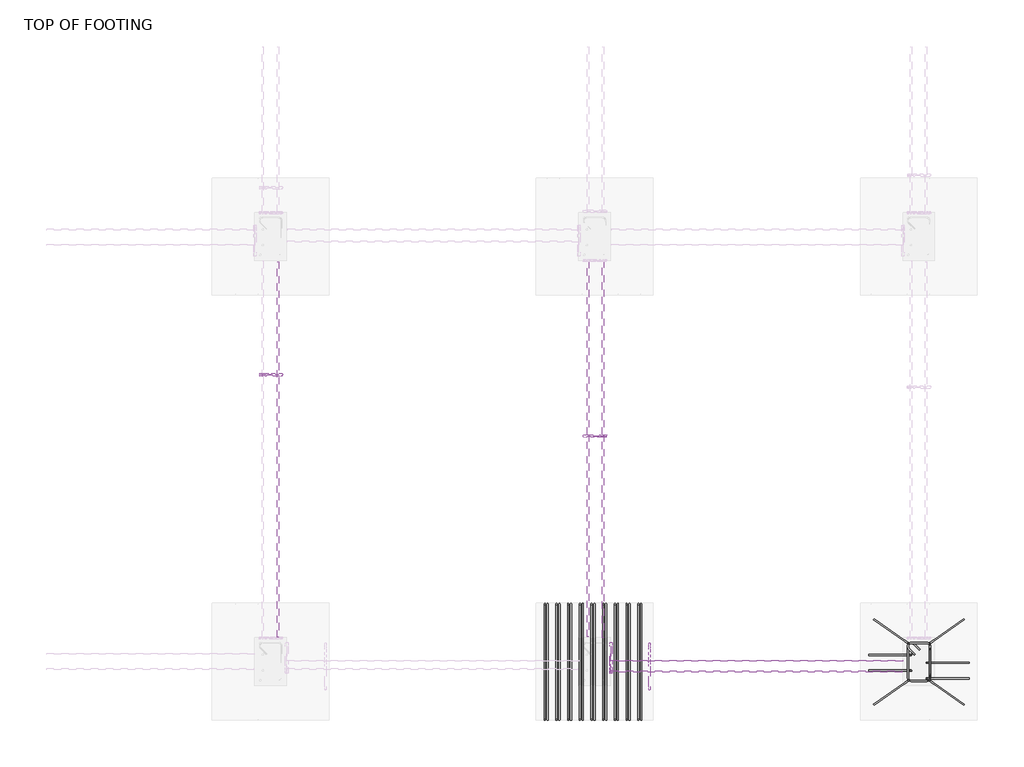
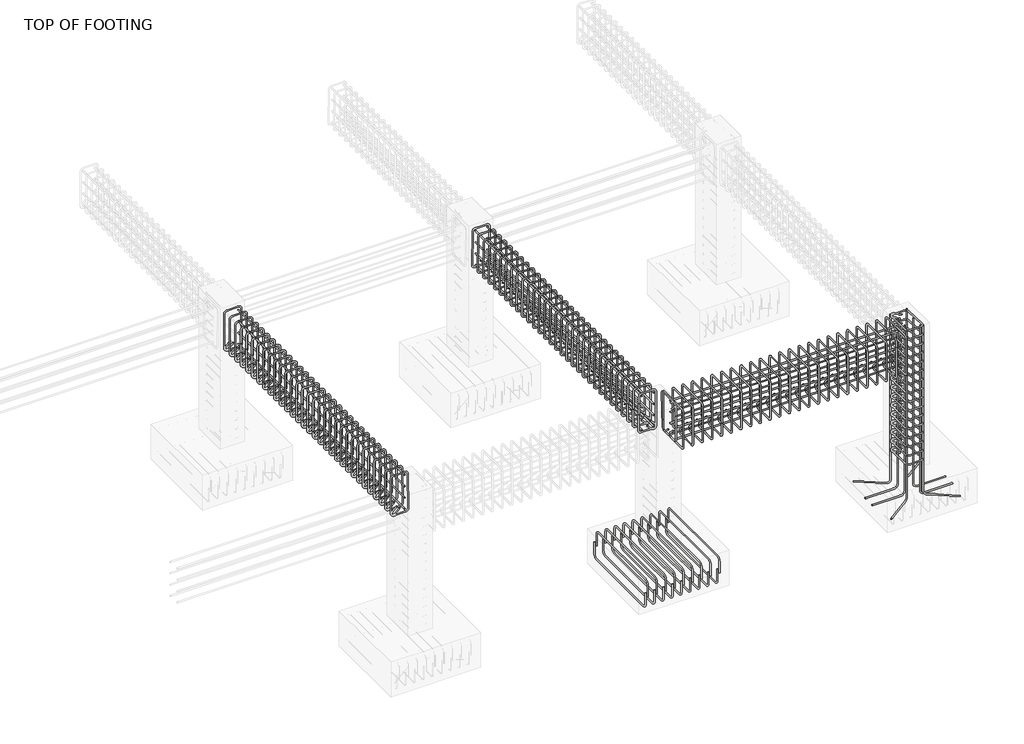
# One storey, part 4 of 18: 18 reinforcing bars.
"""IFC4 building model written with IfcOpenShell, lengths in millimetres."""

from ifc_helpers import new_model, si_unit, point, frame, origin, place, context, project, spatial, polyline, circle_curve, trimmed, segment, composite_curve, source, transform, mapped, element, save
from ifc_brep_helpers import swept_disk

model = new_model("IFC4")

# Units and contexts
model_context = context("Model", 3, world=origin())
ifc_project = project(units=[si_unit("LENGTHUNIT", "METRE", prefix="MILLI")], contexts=[model_context])

# Site, building, storey
site = spatial("IfcSite", under=ifc_project)
building = spatial("IfcBuilding", under=site)
storey = spatial("IfcBuildingStorey", under=building, Name="TOP OF FOOTING", Elevation=-1828.8)

# Reinforcing bars
placement = place(None, origin())
reinforcing_bar_shape = source(origin(), model_context, "Body", "SolidModel", [
    swept_disk(composite_curve([segment(polyline([(-1971.9859643, 5574.8477614, -40.0), (-1971.9859643, 5574.8477614, -2185.2530621)]), True, "CONTINUOUS"), segment(trimmed(circle_curve(frame((-2018.3359643, 5574.8477614, -2185.2530621), z_axis=(0.0, 1.0, 0.0), x_axis=(46.34999999999991, 0.0, 0.0)), 46.35), [point((-1971.9859643, 5574.8477614, -2185.2530621))], [point((-2018.3359643, 5574.8477614, -2231.6030621))], True, "CARTESIAN"), True, "CONTINUOUS"), segment(polyline([(-2018.3359643, 5574.8477614, -2231.6030621), (-2369.5126143, 5574.8477614, -2231.6030621)]), True, "CONTINUOUS")], self_intersect=False), 6.35),
])
element("IfcReinforcingBar", 1, at=placement, inside=storey, context=model_context, shape_type="MappedRepresentation", body=[
    mapped(reinforcing_bar_shape, transform((0.0, 0.0, 0.0), x_axis=(1.0, 0.0, 0.0), y_axis=(0.0, 1.0, 0.0), z_axis=(0.0, 0.0, 1.0))),
    mapped(reinforcing_bar_shape, transform((0.0, 148.3194112, 0.0), x_axis=(1.0, 0.0, 0.0), y_axis=(0.0, 1.0, 0.0), z_axis=(0.0, 0.0, 1.0))),
])
element("IfcReinforcingBar", 2, at=placement, inside=storey, context=model_context, shape_type="SolidModel", body=[
    swept_disk(composite_curve([segment(polyline([(-1996.9859643, 5830.3098681, -40.0), (-1996.9859643, 5830.3098681, -2185.2530621)]), True, "CONTINUOUS"), segment(trimmed(circle_curve(frame((-2034.9536616, 5856.895136, -2185.2530621), z_axis=(0.5735764363510552, 0.8191520442889856, 0.0), x_axis=(37.967697300000054, -26.585267899999963, 0.0)), 46.35), [point((-1996.9859643, 5830.3098681, -2185.2530621))], [point((-2034.9536616, 5856.895136, -2231.6030621))], True, "CARTESIAN"), True, "CONTINUOUS"), segment(polyline([(-2034.9536616, 5856.895136, -2231.6030621), (-2322.6207323, 6058.3217874, -2231.6030621)]), True, "CONTINUOUS")], self_intersect=False), 6.35),
])
reinforcing_bar_2_shape = source(origin(), model_context, "Body", "SolidModel", [
    swept_disk(composite_curve([segment(polyline([(-1892.6954038, 5770.3841028, -1782.45), (-1948.4389667, 5826.1276657, -1782.45)]), True, "CONTINUOUS"), segment(trimmed(circle_curve(frame((-1970.6067643, 5803.9598681, -1782.45), z_axis=(0.0, 0.0, 1.0), x_axis=(22.167797599999858, 22.167797600000085, 0.0)), 31.35), [point((-1948.4389667, 5826.1276657, -1782.45))], [point((-2001.9567643, 5803.9598681, -1782.45))], True, "CARTESIAN"), True, "CONTINUOUS"), segment(polyline([(-2001.9567643, 5803.9598681, -1782.45), (-2001.9567643, 5509.3598681, -1782.45)]), True, "CONTINUOUS"), segment(trimmed(circle_curve(frame((-1970.6067643, 5509.3598681, -1782.45), z_axis=(0.0, 0.0, 1.0), x_axis=(-31.350000000000136, 0.0, 0.0)), 31.35), [point((-2001.9567643, 5509.3598681, -1782.45))], [point((-1970.6067643, 5478.0098681, -1782.45))], True, "CARTESIAN"), True, "CONTINUOUS"), segment(polyline([(-1970.6067643, 5478.0098681, -1782.45), (-1826.0067643, 5478.0098681, -1782.45)]), True, "CONTINUOUS"), segment(trimmed(circle_curve(frame((-1826.0067643, 5509.3400831, -1783.5636125), z_axis=(0.0, 0.0355219283344819, 0.9993688971583016), x_axis=(0.0, -31.330214999999953, 1.1136125000000447)), 31.35), [point((-1826.0067643, 5478.0098681, -1782.45))], [point((-1794.6567643, 5509.3400831, -1783.5636125))], True, "CARTESIAN"), True, "CONTINUOUS"), segment(polyline([(-1794.6567643, 5509.3400831, -1783.5636125), (-1794.6567643, 5803.9796532, -1794.0363875)]), True, "CONTINUOUS"), segment(trimmed(circle_curve(frame((-1826.0067643, 5803.9796532, -1794.0363875), z_axis=(0.0, 0.0355219283344819, 0.9993688971583016), x_axis=(31.34999999999991, 0.0, 0.0)), 31.35), [point((-1794.6567643, 5803.9796532, -1794.0363875))], [point((-1826.0067643, 5835.3098681, -1795.15))], True, "CARTESIAN"), True, "CONTINUOUS"), segment(polyline([(-1826.0067643, 5835.3098681, -1795.15), (-1970.6067643, 5835.3098681, -1795.15)]), True, "CONTINUOUS"), segment(trimmed(circle_curve(frame((-1970.6067643, 5803.9598681, -1795.15), z_axis=(0.0, 0.0, 1.0), x_axis=(0.0, 31.350000000000364, 0.0)), 31.35), [point((-1970.6067643, 5835.3098681, -1795.15))], [point((-1992.7745619, 5781.7920705, -1795.15))], True, "CARTESIAN"), True, "CONTINUOUS"), segment(polyline([(-1992.7745619, 5781.7920705, -1795.15), (-1937.030999, 5726.0485076, -1795.15)]), True, "CONTINUOUS")], self_intersect=False), 6.35),
])
element("IfcReinforcingBar", 3, at=placement, inside=storey, context=model_context, shape_type="MappedRepresentation", body=[
    mapped(reinforcing_bar_2_shape, transform((0.0, 0.0, 0.0), x_axis=(1.0, 0.0, 0.0), y_axis=(0.0, 1.0, 0.0), z_axis=(0.0, 0.0, 1.0))),
    mapped(reinforcing_bar_2_shape, transform((0.0, 0.0, 116.0092918), x_axis=(1.0, 0.0, 0.0), y_axis=(0.0, 1.0, 0.0), z_axis=(0.0, 0.0, 1.0))),
    mapped(reinforcing_bar_2_shape, transform((0.0, 0.0, 232.0185836), x_axis=(1.0, 0.0, 0.0), y_axis=(0.0, 1.0, 0.0), z_axis=(0.0, 0.0, 1.0))),
    mapped(reinforcing_bar_2_shape, transform((0.0, 0.0, 348.0278755), x_axis=(1.0, 0.0, 0.0), y_axis=(0.0, 1.0, 0.0), z_axis=(0.0, 0.0, 1.0))),
    mapped(reinforcing_bar_2_shape, transform((0.0, 0.0, 464.0371673), x_axis=(1.0, 0.0, 0.0), y_axis=(0.0, 1.0, 0.0), z_axis=(0.0, 0.0, 1.0))),
    mapped(reinforcing_bar_2_shape, transform((0.0, 0.0, 580.0464591), x_axis=(1.0, 0.0, 0.0), y_axis=(0.0, 1.0, 0.0), z_axis=(0.0, 0.0, 1.0))),
    mapped(reinforcing_bar_2_shape, transform((0.0, 0.0, 696.0557509), x_axis=(1.0, 0.0, 0.0), y_axis=(0.0, 1.0, 0.0), z_axis=(0.0, 0.0, 1.0))),
    mapped(reinforcing_bar_2_shape, transform((0.0, 0.0, 812.0650428), x_axis=(1.0, 0.0, 0.0), y_axis=(0.0, 1.0, 0.0), z_axis=(0.0, 0.0, 1.0))),
    mapped(reinforcing_bar_2_shape, transform((0.0, 0.0, 928.0743346), x_axis=(1.0, 0.0, 0.0), y_axis=(0.0, 1.0, 0.0), z_axis=(0.0, 0.0, 1.0))),
    mapped(reinforcing_bar_2_shape, transform((0.0, 0.0, 1044.0836264), x_axis=(1.0, 0.0, 0.0), y_axis=(0.0, 1.0, 0.0), z_axis=(0.0, 0.0, 1.0))),
    mapped(reinforcing_bar_2_shape, transform((0.0, 0.0, 1160.0929182), x_axis=(1.0, 0.0, 0.0), y_axis=(0.0, 1.0, 0.0), z_axis=(0.0, 0.0, 1.0))),
    mapped(reinforcing_bar_2_shape, transform((0.0, 0.0, 1276.1022101), x_axis=(1.0, 0.0, 0.0), y_axis=(0.0, 1.0, 0.0), z_axis=(0.0, 0.0, 1.0))),
    mapped(reinforcing_bar_2_shape, transform((0.0, 0.0, 1392.1115019), x_axis=(1.0, 0.0, 0.0), y_axis=(0.0, 1.0, 0.0), z_axis=(0.0, 0.0, 1.0))),
    mapped(reinforcing_bar_2_shape, transform((0.0, 0.0, 1508.1207937), x_axis=(1.0, 0.0, 0.0), y_axis=(0.0, 1.0, 0.0), z_axis=(0.0, 0.0, 1.0))),
    mapped(reinforcing_bar_2_shape, transform((0.0, 0.0, 1624.1300855), x_axis=(1.0, 0.0, 0.0), y_axis=(0.0, 1.0, 0.0), z_axis=(0.0, 0.0, 1.0))),
    mapped(reinforcing_bar_2_shape, transform((0.0, 0.0, 1740.1393774), x_axis=(1.0, 0.0, 0.0), y_axis=(0.0, 1.0, 0.0), z_axis=(0.0, 0.0, 1.0))),
])
element("IfcReinforcingBar", 4, at=placement, inside=storey, context=model_context, shape_type="SolidModel", body=[
    swept_disk(composite_curve([segment(polyline([(-1799.6275643, 5830.3098681, -40.0), (-1799.6275643, 5830.3098681, -2185.2530621)]), True, "CONTINUOUS"), segment(trimmed(circle_curve(frame((-1761.6598671, 5856.895136, -2185.2530621), z_axis=(0.5735764363510552, -0.8191520442889856, 0.0), x_axis=(-37.967697199999975, -26.585267899999963, 0.0)), 46.35), [point((-1799.6275643, 5830.3098681, -2185.2530621))], [point((-1761.6598671, 5856.895136, -2231.6030621))], True, "CARTESIAN"), True, "CONTINUOUS"), segment(polyline([(-1761.6598671, 5856.895136, -2231.6030621), (-1473.9927964, 6058.3217874, -2231.6030621)]), True, "CONTINUOUS")], self_intersect=False), 6.35),
])
element("IfcReinforcingBar", 5, at=placement, inside=storey, context=model_context, shape_type="SolidModel", body=[
    swept_disk(composite_curve([segment(polyline([(-1996.9859643, 5483.0098681, -40.0), (-1996.9859643, 5483.0098681, -2185.2530621)]), True, "CONTINUOUS"), segment(trimmed(circle_curve(frame((-2034.9536616, 5456.4246003, -2185.2530621), z_axis=(-0.5735764363510106, 0.8191520442890167, 0.0), x_axis=(37.967697300000054, 26.58526780000011, 0.0)), 46.35), [point((-1996.9859643, 5483.0098681, -2185.2530621))], [point((-2034.9536616, 5456.4246003, -2231.6030621))], True, "CARTESIAN"), True, "CONTINUOUS"), segment(polyline([(-2034.9536616, 5456.4246003, -2231.6030621), (-2322.6207323, 5254.9979489, -2231.6030621)]), True, "CONTINUOUS")], self_intersect=False), 6.35),
])
element("IfcReinforcingBar", 6, at=placement, inside=storey, context=model_context, shape_type="SolidModel", body=[
    swept_disk(composite_curve([segment(polyline([(-1799.6275643, 5483.0098681, -40.0), (-1799.6275643, 5483.0098681, -2185.2530621)]), True, "CONTINUOUS"), segment(trimmed(circle_curve(frame((-1761.6598671, 5456.4246003, -2185.2530621), z_axis=(-0.5735764363510997, -0.8191520442889543, 0.0), x_axis=(-37.967697199999975, 26.58526780000011, 0.0)), 46.35), [point((-1799.6275643, 5483.0098681, -2185.2530621))], [point((-1761.6598671, 5456.4246003, -2231.6030621))], True, "CARTESIAN"), True, "CONTINUOUS"), segment(polyline([(-1761.6598671, 5456.4246003, -2231.6030621), (-1473.9927964, 5254.9979489, -2231.6030621)]), True, "CONTINUOUS")], self_intersect=False), 6.35),
])
reinforcing_bar_3_shape = source(origin(), model_context, "Body", "SolidModel", [
    swept_disk(composite_curve([segment(polyline([(-1824.6275643, 5499.8477614, -40.0), (-1824.6275643, 5499.8477614, -2185.2530621)]), True, "CONTINUOUS"), segment(trimmed(circle_curve(frame((-1778.2775643, 5499.8477614, -2185.2530621), z_axis=(0.0, -1.0, 0.0), x_axis=(-46.34999999999991, 0.0, 0.0)), 46.35), [point((-1824.6275643, 5499.8477614, -2185.2530621))], [point((-1778.2775643, 5499.8477614, -2231.6030621))], True, "CARTESIAN"), True, "CONTINUOUS"), segment(polyline([(-1778.2775643, 5499.8477614, -2231.6030621), (-1427.1009144, 5499.8477614, -2231.6030621)]), True, "CONTINUOUS")], self_intersect=False), 6.35),
])
element("IfcReinforcingBar", 7, at=placement, inside=storey, context=model_context, shape_type="MappedRepresentation", body=[
    mapped(reinforcing_bar_3_shape, transform((0.0, 0.0, 0.0), x_axis=(1.0, 0.0, 0.0), y_axis=(0.0, 1.0, 0.0), z_axis=(0.0, 0.0, 1.0))),
    mapped(reinforcing_bar_3_shape, transform((0.0, 148.3194112, 0.0), x_axis=(1.0, 0.0, 0.0), y_axis=(0.0, 1.0, 0.0), z_axis=(0.0, 0.0, 1.0))),
])
reinforcing_bar_4_shape = source(origin(), model_context, "Body", "SolidModel", [
    swept_disk(composite_curve([segment(polyline([(-4511.1065918, 6200.3098681, -2080.1793981), (-4511.1065918, 6200.3098681, -1932.8793981)]), True, "CONTINUOUS"), segment(trimmed(circle_curve(frame((-4511.1065918, 6153.9598681, -1932.8793981), z_axis=(1.0, 0.0, 0.0), x_axis=(0.0, 46.350000000000364, 0.0)), 46.35), [point((-4511.1065918, 6200.3098681, -1932.8793981))], [point((-4511.1065918, 6153.9598681, -1886.5293981))], True, "CARTESIAN"), True, "CONTINUOUS"), segment(polyline([(-4511.1065918, 6153.9598681, -1886.5293981), (-4511.1065918, 5159.3598681, -1886.5293981)]), True, "CONTINUOUS"), segment(trimmed(circle_curve(frame((-4511.1065918, 5159.3598681, -1932.8793981), z_axis=(1.0, 0.0, 0.0), x_axis=(0.0, 0.0, 46.34999999999991)), 46.35), [point((-4511.1065918, 5159.3598681, -1886.5293981))], [point((-4511.1065918, 5113.0098681, -1932.8793981))], True, "CARTESIAN"), True, "CONTINUOUS"), segment(polyline([(-4511.1065918, 5113.0098681, -1932.8793981), (-4511.1065918, 5113.0098681, -2080.1793981)]), True, "CONTINUOUS")], self_intersect=False), 6.35),
])
element("IfcReinforcingBar", 8, at=placement, inside=storey, context=model_context, shape_type="MappedRepresentation", body=[
    mapped(reinforcing_bar_4_shape, transform((0.0, 0.0, 0.0), x_axis=(1.0, 0.0, 0.0), y_axis=(0.0, 1.0, 0.0), z_axis=(0.0, 0.0, 1.0))),
    mapped(reinforcing_bar_4_shape, transform((-109.9785589, 0.0, 0.0), x_axis=(1.0, 0.0, 0.0), y_axis=(0.0, 1.0, 0.0), z_axis=(0.0, 0.0, 1.0))),
    mapped(reinforcing_bar_4_shape, transform((-219.9571177, 0.0, 0.0), x_axis=(1.0, 0.0, 0.0), y_axis=(0.0, 1.0, 0.0), z_axis=(0.0, 0.0, 1.0))),
    mapped(reinforcing_bar_4_shape, transform((-329.9356766, 0.0, 0.0), x_axis=(1.0, 0.0, 0.0), y_axis=(0.0, 1.0, 0.0), z_axis=(0.0, 0.0, 1.0))),
    mapped(reinforcing_bar_4_shape, transform((-439.9142355, 0.0, 0.0), x_axis=(1.0, 0.0, 0.0), y_axis=(0.0, 1.0, 0.0), z_axis=(0.0, 0.0, 1.0))),
    mapped(reinforcing_bar_4_shape, transform((-549.8927943, 0.0, 0.0), x_axis=(1.0, 0.0, 0.0), y_axis=(0.0, 1.0, 0.0), z_axis=(0.0, 0.0, 1.0))),
    mapped(reinforcing_bar_4_shape, transform((-659.8713532, 0.0, 0.0), x_axis=(1.0, 0.0, 0.0), y_axis=(0.0, 1.0, 0.0), z_axis=(0.0, 0.0, 1.0))),
    mapped(reinforcing_bar_4_shape, transform((-769.8499121, 0.0, 0.0), x_axis=(1.0, 0.0, 0.0), y_axis=(0.0, 1.0, 0.0), z_axis=(0.0, 0.0, 1.0))),
    mapped(reinforcing_bar_4_shape, transform((-879.828471, 0.0, 0.0), x_axis=(1.0, 0.0, 0.0), y_axis=(0.0, 1.0, 0.0), z_axis=(0.0, 0.0, 1.0))),
])
reinforcing_bar_5_shape = source(origin(), model_context, "Body", "SolidModel", [
    swept_disk(composite_curve([segment(polyline([(-5417.5126143, 6200.3098681, -2025.2530621), (-5417.5126143, 6200.3098681, -2172.5530621)]), True, "CONTINUOUS"), segment(trimmed(circle_curve(frame((-5417.5126143, 6153.9598681, -2172.5530621), z_axis=(-1.0, 0.0, 0.0), x_axis=(0.0, 46.350000000000364, 0.0)), 46.35), [point((-5417.5126143, 6200.3098681, -2172.5530621))], [point((-5417.5126143, 6153.9598681, -2218.9030621))], True, "CARTESIAN"), True, "CONTINUOUS"), segment(polyline([(-5417.5126143, 6153.9598681, -2218.9030621), (-5417.5126143, 5159.3598681, -2218.9030621)]), True, "CONTINUOUS"), segment(trimmed(circle_curve(frame((-5417.5126143, 5159.3598681, -2172.5530621), z_axis=(-1.0, 0.0, 0.0), x_axis=(0.0, 0.0, -46.350000000000364)), 46.35), [point((-5417.5126143, 5159.3598681, -2218.9030621))], [point((-5417.5126143, 5113.0098681, -2172.5530621))], True, "CARTESIAN"), True, "CONTINUOUS"), segment(polyline([(-5417.5126143, 5113.0098681, -2172.5530621), (-5417.5126143, 5113.0098681, -2025.2530621)]), True, "CONTINUOUS")], self_intersect=False), 6.35),
])
element("IfcReinforcingBar", 9, at=placement, inside=storey, context=model_context, shape_type="MappedRepresentation", body=[
    mapped(reinforcing_bar_5_shape, transform((0.0, 0.0, 0.0), x_axis=(1.0, 0.0, 0.0), y_axis=(0.0, 1.0, 0.0), z_axis=(0.0, 0.0, 1.0))),
    mapped(reinforcing_bar_5_shape, transform((109.9890349, 0.0, 0.0), x_axis=(1.0, 0.0, 0.0), y_axis=(0.0, 1.0, 0.0), z_axis=(0.0, 0.0, 1.0))),
    mapped(reinforcing_bar_5_shape, transform((219.9780699, 0.0, 0.0), x_axis=(1.0, 0.0, 0.0), y_axis=(0.0, 1.0, 0.0), z_axis=(0.0, 0.0, 1.0))),
    mapped(reinforcing_bar_5_shape, transform((329.9671048, 0.0, 0.0), x_axis=(1.0, 0.0, 0.0), y_axis=(0.0, 1.0, 0.0), z_axis=(0.0, 0.0, 1.0))),
    mapped(reinforcing_bar_5_shape, transform((439.9561397, 0.0, 0.0), x_axis=(1.0, 0.0, 0.0), y_axis=(0.0, 1.0, 0.0), z_axis=(0.0, 0.0, 1.0))),
    mapped(reinforcing_bar_5_shape, transform((549.9451746, 0.0, 0.0), x_axis=(1.0, 0.0, 0.0), y_axis=(0.0, 1.0, 0.0), z_axis=(0.0, 0.0, 1.0))),
    mapped(reinforcing_bar_5_shape, transform((659.9342096, 0.0, 0.0), x_axis=(1.0, 0.0, 0.0), y_axis=(0.0, 1.0, 0.0), z_axis=(0.0, 0.0, 1.0))),
    mapped(reinforcing_bar_5_shape, transform((769.9232445, 0.0, 0.0), x_axis=(1.0, 0.0, 0.0), y_axis=(0.0, 1.0, 0.0), z_axis=(0.0, 0.0, 1.0))),
    mapped(reinforcing_bar_5_shape, transform((879.9122794, 0.0, 0.0), x_axis=(1.0, 0.0, 0.0), y_axis=(0.0, 1.0, 0.0), z_axis=(0.0, 0.0, 1.0))),
])
reinforcing_bar_6_shape = source(origin(), model_context, "Body", "SolidModel", [
    swept_disk(composite_curve([segment(polyline([(-7988.6954038, 5888.0098675, -488.7242346), (-8044.4389667, 5888.0098675, -544.4677976)]), True, "CONTINUOUS"), segment(trimmed(circle_curve(frame((-8066.6067643, 5888.0098675, -522.3), z_axis=(0.0, 1.0, 0.0), x_axis=(22.167797600000085, 0.0, -22.167797600000085)), 31.35), [point((-8044.4389667, 5888.0098675, -544.4677976))], [point((-8097.9567643, 5888.0098675, -522.3))], True, "CARTESIAN"), True, "CONTINUOUS"), segment(polyline([(-8097.9567643, 5888.0098675, -522.3), (-8097.9567643, 5888.0098675, -77.7)]), True, "CONTINUOUS"), segment(trimmed(circle_curve(frame((-8066.6067643, 5888.0098675, -77.7), z_axis=(0.0, 1.0, 0.0), x_axis=(-31.350000000000364, 0.0, 0.0)), 31.35), [point((-8097.9567643, 5888.0098675, -77.7))], [point((-8066.6067643, 5888.0098675, -46.35))], True, "CARTESIAN"), True, "CONTINUOUS"), segment(polyline([(-8066.6067643, 5888.0098675, -46.35), (-7922.0067643, 5888.0098675, -46.35)]), True, "CONTINUOUS"), segment(trimmed(circle_curve(frame((-7922.0067643, 5887.2252819, -77.6901807), z_axis=(0.0, 0.9996867842138424, -0.025026655153786322), x_axis=(0.0, 0.784585600000355, 31.340180699999998)), 31.35), [point((-7922.0067643, 5888.0098675, -46.35))], [point((-7890.6567643, 5887.2252819, -77.6901807))], True, "CARTESIAN"), True, "CONTINUOUS"), segment(polyline([(-7890.6567643, 5887.2252819, -77.6901807), (-7890.6567643, 5876.0944532, -522.3098193)]), True, "CONTINUOUS"), segment(trimmed(circle_curve(frame((-7922.0067643, 5876.0944532, -522.3098193), z_axis=(0.0, 0.9996867842138424, -0.025026655153786322), x_axis=(31.350000000000364, 0.0, 0.0)), 31.35), [point((-7890.6567643, 5876.0944532, -522.3098193))], [point((-7922.0067643, 5875.3098675, -553.65))], True, "CARTESIAN"), True, "CONTINUOUS"), segment(polyline([(-7922.0067643, 5875.3098675, -553.65), (-8066.6067643, 5875.3098675, -553.65)]), True, "CONTINUOUS"), segment(trimmed(circle_curve(frame((-8066.6067643, 5875.3098675, -522.3), z_axis=(0.0, 1.0, 0.0), x_axis=(0.0, 0.0, -31.350000000000023)), 31.35), [point((-8066.6067643, 5875.3098675, -553.65))], [point((-8088.7745619, 5875.3098675, -500.1322024))], True, "CARTESIAN"), True, "CONTINUOUS"), segment(polyline([(-8088.7745619, 5875.3098675, -500.1322024), (-8033.030999, 5875.3098675, -444.3886395)]), True, "CONTINUOUS")], self_intersect=False), 6.35),
])
element("IfcReinforcingBar", 10, at=placement, inside=storey, context=model_context, shape_type="MappedRepresentation", body=[
    mapped(reinforcing_bar_6_shape, transform((0.0, 0.0, 0.0), x_axis=(1.0, 0.0, 0.0), y_axis=(0.0, 1.0, 0.0), z_axis=(0.0, 0.0, 1.0))),
    mapped(reinforcing_bar_6_shape, transform((0.0, 117.91, 0.0), x_axis=(1.0, 0.0, 0.0), y_axis=(0.0, 1.0, 0.0), z_axis=(0.0, 0.0, 1.0))),
    mapped(reinforcing_bar_6_shape, transform((0.0, 235.82, 0.0), x_axis=(1.0, 0.0, 0.0), y_axis=(0.0, 1.0, 0.0), z_axis=(0.0, 0.0, 1.0))),
    mapped(reinforcing_bar_6_shape, transform((0.0, 353.7300001, 0.0), x_axis=(1.0, 0.0, 0.0), y_axis=(0.0, 1.0, 0.0), z_axis=(0.0, 0.0, 1.0))),
    mapped(reinforcing_bar_6_shape, transform((0.0, 471.6400001, 0.0), x_axis=(1.0, 0.0, 0.0), y_axis=(0.0, 1.0, 0.0), z_axis=(0.0, 0.0, 1.0))),
    mapped(reinforcing_bar_6_shape, transform((0.0, 589.5500001, 0.0), x_axis=(1.0, 0.0, 0.0), y_axis=(0.0, 1.0, 0.0), z_axis=(0.0, 0.0, 1.0))),
    mapped(reinforcing_bar_6_shape, transform((0.0, 707.4600001, 0.0), x_axis=(1.0, 0.0, 0.0), y_axis=(0.0, 1.0, 0.0), z_axis=(0.0, 0.0, 1.0))),
    mapped(reinforcing_bar_6_shape, transform((0.0, 825.3700001, 0.0), x_axis=(1.0, 0.0, 0.0), y_axis=(0.0, 1.0, 0.0), z_axis=(0.0, 0.0, 1.0))),
    mapped(reinforcing_bar_6_shape, transform((0.0, 943.2800002, 0.0), x_axis=(1.0, 0.0, 0.0), y_axis=(0.0, 1.0, 0.0), z_axis=(0.0, 0.0, 1.0))),
    mapped(reinforcing_bar_6_shape, transform((0.0, 1061.1900002, 0.0), x_axis=(1.0, 0.0, 0.0), y_axis=(0.0, 1.0, 0.0), z_axis=(0.0, 0.0, 1.0))),
    mapped(reinforcing_bar_6_shape, transform((0.0, 1179.1000002, 0.0), x_axis=(1.0, 0.0, 0.0), y_axis=(0.0, 1.0, 0.0), z_axis=(0.0, 0.0, 1.0))),
    mapped(reinforcing_bar_6_shape, transform((0.0, 1297.0100002, 0.0), x_axis=(1.0, 0.0, 0.0), y_axis=(0.0, 1.0, 0.0), z_axis=(0.0, 0.0, 1.0))),
    mapped(reinforcing_bar_6_shape, transform((0.0, 1414.9200002, 0.0), x_axis=(1.0, 0.0, 0.0), y_axis=(0.0, 1.0, 0.0), z_axis=(0.0, 0.0, 1.0))),
    mapped(reinforcing_bar_6_shape, transform((0.0, 1532.8300003, 0.0), x_axis=(1.0, 0.0, 0.0), y_axis=(0.0, 1.0, 0.0), z_axis=(0.0, 0.0, 1.0))),
    mapped(reinforcing_bar_6_shape, transform((0.0, 1650.7400003, 0.0), x_axis=(1.0, 0.0, 0.0), y_axis=(0.0, 1.0, 0.0), z_axis=(0.0, 0.0, 1.0))),
    mapped(reinforcing_bar_6_shape, transform((0.0, 1768.6500003, 0.0), x_axis=(1.0, 0.0, 0.0), y_axis=(0.0, 1.0, 0.0), z_axis=(0.0, 0.0, 1.0))),
    mapped(reinforcing_bar_6_shape, transform((0.0, 1886.5600003, 0.0), x_axis=(1.0, 0.0, 0.0), y_axis=(0.0, 1.0, 0.0), z_axis=(0.0, 0.0, 1.0))),
    mapped(reinforcing_bar_6_shape, transform((0.0, 2004.4700003, 0.0), x_axis=(1.0, 0.0, 0.0), y_axis=(0.0, 1.0, 0.0), z_axis=(0.0, 0.0, 1.0))),
    mapped(reinforcing_bar_6_shape, transform((0.0, 2122.3800004, 0.0), x_axis=(1.0, 0.0, 0.0), y_axis=(0.0, 1.0, 0.0), z_axis=(0.0, 0.0, 1.0))),
    mapped(reinforcing_bar_6_shape, transform((0.0, 2240.2900004, 0.0), x_axis=(1.0, 0.0, 0.0), y_axis=(0.0, 1.0, 0.0), z_axis=(0.0, 0.0, 1.0))),
    mapped(reinforcing_bar_6_shape, transform((0.0, 2358.2000004, 0.0), x_axis=(1.0, 0.0, 0.0), y_axis=(0.0, 1.0, 0.0), z_axis=(0.0, 0.0, 1.0))),
    mapped(reinforcing_bar_6_shape, transform((0.0, 2476.1100004, 0.0), x_axis=(1.0, 0.0, 0.0), y_axis=(0.0, 1.0, 0.0), z_axis=(0.0, 0.0, 1.0))),
    mapped(reinforcing_bar_6_shape, transform((0.0, 2594.0200004, 0.0), x_axis=(1.0, 0.0, 0.0), y_axis=(0.0, 1.0, 0.0), z_axis=(0.0, 0.0, 1.0))),
    mapped(reinforcing_bar_6_shape, transform((0.0, 2711.9300005, 0.0), x_axis=(1.0, 0.0, 0.0), y_axis=(0.0, 1.0, 0.0), z_axis=(0.0, 0.0, 1.0))),
    mapped(reinforcing_bar_6_shape, transform((0.0, 2829.8400005, 0.0), x_axis=(1.0, 0.0, 0.0), y_axis=(0.0, 1.0, 0.0), z_axis=(0.0, 0.0, 1.0))),
    mapped(reinforcing_bar_6_shape, transform((0.0, 2947.7500005, 0.0), x_axis=(1.0, 0.0, 0.0), y_axis=(0.0, 1.0, 0.0), z_axis=(0.0, 0.0, 1.0))),
    mapped(reinforcing_bar_6_shape, transform((0.0, 3065.6600005, 0.0), x_axis=(1.0, 0.0, 0.0), y_axis=(0.0, 1.0, 0.0), z_axis=(0.0, 0.0, 1.0))),
    mapped(reinforcing_bar_6_shape, transform((0.0, 3183.5700005, 0.0), x_axis=(1.0, 0.0, 0.0), y_axis=(0.0, 1.0, 0.0), z_axis=(0.0, 0.0, 1.0))),
    mapped(reinforcing_bar_6_shape, transform((0.0, 3301.4800006, 0.0), x_axis=(1.0, 0.0, 0.0), y_axis=(0.0, 1.0, 0.0), z_axis=(0.0, 0.0, 1.0))),
    mapped(reinforcing_bar_6_shape, transform((0.0, 3419.3900006, 0.0), x_axis=(1.0, 0.0, 0.0), y_axis=(0.0, 1.0, 0.0), z_axis=(0.0, 0.0, 1.0))),
    mapped(reinforcing_bar_6_shape, transform((0.0, 3537.3000006, 0.0), x_axis=(1.0, 0.0, 0.0), y_axis=(0.0, 1.0, 0.0), z_axis=(0.0, 0.0, 1.0))),
])
reinforcing_bar_7_shape = source(origin(), model_context, "Body", "SolidModel", [
    swept_disk(composite_curve([segment(polyline([(-7928.3740978, 5886.6742321, -524.1097861), (-7928.3740978, 9421.3452184, -524.1097861)]), True, "CONTINUOUS")], self_intersect=False), 6.35),
])
element("IfcReinforcingBar", 11, at=placement, inside=storey, context=model_context, shape_type="MappedRepresentation", body=[
    mapped(reinforcing_bar_7_shape, transform((0.0, 0.0, 0.0), x_axis=(1.0, 0.0, 0.0), y_axis=(0.0, 1.0, 0.0), z_axis=(0.0, 0.0, 1.0))),
    mapped(reinforcing_bar_7_shape, transform((0.0, 0.0, 147.1005596), x_axis=(1.0, 0.0, 0.0), y_axis=(0.0, 1.0, 0.0), z_axis=(0.0, 0.0, 1.0))),
    mapped(reinforcing_bar_7_shape, transform((0.0, 0.0, 294.2011193), x_axis=(1.0, 0.0, 0.0), y_axis=(0.0, 1.0, 0.0), z_axis=(0.0, 0.0, 1.0))),
    mapped(reinforcing_bar_7_shape, transform((0.0, 0.0, 441.3016789), x_axis=(1.0, 0.0, 0.0), y_axis=(0.0, 1.0, 0.0), z_axis=(0.0, 0.0, 1.0))),
])
reinforcing_bar_8_shape = source(origin(), model_context, "Body", "SolidModel", [
    swept_disk(composite_curve([segment(polyline([(-4951.9181249, 9425.3098681, -488.7242346), (-4896.1745619, 9425.3098681, -544.4677976)]), True, "CONTINUOUS"), segment(trimmed(circle_curve(frame((-4874.0067643, 9425.3098681, -522.3), z_axis=(0.0, -1.0, 0.0), x_axis=(-22.167797600000085, 0.0, -22.167797600000085)), 31.35), [point((-4896.1745619, 9425.3098681, -544.4677976))], [point((-4842.6567643, 9425.3098681, -522.3))], True, "CARTESIAN"), True, "CONTINUOUS"), segment(polyline([(-4842.6567643, 9425.3098681, -522.3), (-4842.6567643, 9425.3098681, -77.7)]), True, "CONTINUOUS"), segment(trimmed(circle_curve(frame((-4874.0067643, 9425.3098681, -77.7), z_axis=(0.0, -1.0, 0.0), x_axis=(31.350000000000364, 0.0, 0.0)), 31.35), [point((-4842.6567643, 9425.3098681, -77.7))], [point((-4874.0067643, 9425.3098681, -46.35))], True, "CARTESIAN"), True, "CONTINUOUS"), segment(polyline([(-4874.0067643, 9425.3098681, -46.35), (-5018.6067643, 9425.3098681, -46.35)]), True, "CONTINUOUS"), segment(trimmed(circle_curve(frame((-5018.6067643, 9426.0944538, -77.6901807), z_axis=(0.0, -0.9996867842138424, -0.025026655153786322), x_axis=(0.0, -0.7845857000011165, 31.340180699999998)), 31.35), [point((-5018.6067643, 9425.3098681, -46.35))], [point((-5049.9567643, 9426.0944538, -77.6901807))], True, "CARTESIAN"), True, "CONTINUOUS"), segment(polyline([(-5049.9567643, 9426.0944538, -77.6901807), (-5049.9567643, 9437.2252825, -522.3098193)]), True, "CONTINUOUS"), segment(trimmed(circle_curve(frame((-5018.6067643, 9437.2252825, -522.3098193), z_axis=(0.0, -0.9996867842138424, -0.025026655153786322), x_axis=(-31.350000000000364, 0.0, 0.0)), 31.35), [point((-5049.9567643, 9437.2252825, -522.3098193))], [point((-5018.6067643, 9438.0098681, -553.65))], True, "CARTESIAN"), True, "CONTINUOUS"), segment(polyline([(-5018.6067643, 9438.0098681, -553.65), (-4874.0067643, 9438.0098681, -553.65)]), True, "CONTINUOUS"), segment(trimmed(circle_curve(frame((-4874.0067643, 9438.0098681, -522.3), z_axis=(0.0, -1.0, 0.0), x_axis=(0.0, 0.0, -31.350000000000023)), 31.35), [point((-4874.0067643, 9438.0098681, -553.65))], [point((-4851.8389667, 9438.0098681, -500.1322024))], True, "CARTESIAN"), True, "CONTINUOUS"), segment(polyline([(-4851.8389667, 9438.0098681, -500.1322024), (-4907.5825297, 9438.0098681, -444.3886395)]), True, "CONTINUOUS")], self_intersect=False), 6.35),
])
element("IfcReinforcingBar", 12, at=placement, inside=storey, context=model_context, shape_type="MappedRepresentation", body=[
    mapped(reinforcing_bar_8_shape, transform((0.0, 0.0, 0.0), x_axis=(1.0, 0.0, 0.0), y_axis=(0.0, 1.0, 0.0), z_axis=(0.0, 0.0, 1.0))),
    mapped(reinforcing_bar_8_shape, transform((0.0, -117.91, 0.0), x_axis=(1.0, 0.0, 0.0), y_axis=(0.0, 1.0, 0.0), z_axis=(0.0, 0.0, 1.0))),
    mapped(reinforcing_bar_8_shape, transform((0.0, -235.82, 0.0), x_axis=(1.0, 0.0, 0.0), y_axis=(0.0, 1.0, 0.0), z_axis=(0.0, 0.0, 1.0))),
    mapped(reinforcing_bar_8_shape, transform((0.0, -353.7300001, 0.0), x_axis=(1.0, 0.0, 0.0), y_axis=(0.0, 1.0, 0.0), z_axis=(0.0, 0.0, 1.0))),
    mapped(reinforcing_bar_8_shape, transform((0.0, -471.6400001, 0.0), x_axis=(1.0, 0.0, 0.0), y_axis=(0.0, 1.0, 0.0), z_axis=(0.0, 0.0, 1.0))),
    mapped(reinforcing_bar_8_shape, transform((0.0, -589.5500001, 0.0), x_axis=(1.0, 0.0, 0.0), y_axis=(0.0, 1.0, 0.0), z_axis=(0.0, 0.0, 1.0))),
    mapped(reinforcing_bar_8_shape, transform((0.0, -707.4600001, 0.0), x_axis=(1.0, 0.0, 0.0), y_axis=(0.0, 1.0, 0.0), z_axis=(0.0, 0.0, 1.0))),
    mapped(reinforcing_bar_8_shape, transform((0.0, -825.3700001, 0.0), x_axis=(1.0, 0.0, 0.0), y_axis=(0.0, 1.0, 0.0), z_axis=(0.0, 0.0, 1.0))),
    mapped(reinforcing_bar_8_shape, transform((0.0, -943.2800002, 0.0), x_axis=(1.0, 0.0, 0.0), y_axis=(0.0, 1.0, 0.0), z_axis=(0.0, 0.0, 1.0))),
    mapped(reinforcing_bar_8_shape, transform((0.0, -1061.1900002, 0.0), x_axis=(1.0, 0.0, 0.0), y_axis=(0.0, 1.0, 0.0), z_axis=(0.0, 0.0, 1.0))),
    mapped(reinforcing_bar_8_shape, transform((0.0, -1179.1000002, 0.0), x_axis=(1.0, 0.0, 0.0), y_axis=(0.0, 1.0, 0.0), z_axis=(0.0, 0.0, 1.0))),
    mapped(reinforcing_bar_8_shape, transform((0.0, -1297.0100002, 0.0), x_axis=(1.0, 0.0, 0.0), y_axis=(0.0, 1.0, 0.0), z_axis=(0.0, 0.0, 1.0))),
    mapped(reinforcing_bar_8_shape, transform((0.0, -1414.9200002, 0.0), x_axis=(1.0, 0.0, 0.0), y_axis=(0.0, 1.0, 0.0), z_axis=(0.0, 0.0, 1.0))),
    mapped(reinforcing_bar_8_shape, transform((0.0, -1532.8300003, 0.0), x_axis=(1.0, 0.0, 0.0), y_axis=(0.0, 1.0, 0.0), z_axis=(0.0, 0.0, 1.0))),
    mapped(reinforcing_bar_8_shape, transform((0.0, -1650.7400003, 0.0), x_axis=(1.0, 0.0, 0.0), y_axis=(0.0, 1.0, 0.0), z_axis=(0.0, 0.0, 1.0))),
    mapped(reinforcing_bar_8_shape, transform((0.0, -1768.6500003, 0.0), x_axis=(1.0, 0.0, 0.0), y_axis=(0.0, 1.0, 0.0), z_axis=(0.0, 0.0, 1.0))),
    mapped(reinforcing_bar_8_shape, transform((0.0, -1886.5600003, 0.0), x_axis=(1.0, 0.0, 0.0), y_axis=(0.0, 1.0, 0.0), z_axis=(0.0, 0.0, 1.0))),
    mapped(reinforcing_bar_8_shape, transform((0.0, -2004.4700003, 0.0), x_axis=(1.0, 0.0, 0.0), y_axis=(0.0, 1.0, 0.0), z_axis=(0.0, 0.0, 1.0))),
    mapped(reinforcing_bar_8_shape, transform((0.0, -2122.3800004, 0.0), x_axis=(1.0, 0.0, 0.0), y_axis=(0.0, 1.0, 0.0), z_axis=(0.0, 0.0, 1.0))),
    mapped(reinforcing_bar_8_shape, transform((0.0, -2240.2900004, 0.0), x_axis=(1.0, 0.0, 0.0), y_axis=(0.0, 1.0, 0.0), z_axis=(0.0, 0.0, 1.0))),
    mapped(reinforcing_bar_8_shape, transform((0.0, -2358.2000004, 0.0), x_axis=(1.0, 0.0, 0.0), y_axis=(0.0, 1.0, 0.0), z_axis=(0.0, 0.0, 1.0))),
    mapped(reinforcing_bar_8_shape, transform((0.0, -2476.1100004, 0.0), x_axis=(1.0, 0.0, 0.0), y_axis=(0.0, 1.0, 0.0), z_axis=(0.0, 0.0, 1.0))),
    mapped(reinforcing_bar_8_shape, transform((0.0, -2594.0200004, 0.0), x_axis=(1.0, 0.0, 0.0), y_axis=(0.0, 1.0, 0.0), z_axis=(0.0, 0.0, 1.0))),
    mapped(reinforcing_bar_8_shape, transform((0.0, -2711.9300005, 0.0), x_axis=(1.0, 0.0, 0.0), y_axis=(0.0, 1.0, 0.0), z_axis=(0.0, 0.0, 1.0))),
    mapped(reinforcing_bar_8_shape, transform((0.0, -2829.8400005, 0.0), x_axis=(1.0, 0.0, 0.0), y_axis=(0.0, 1.0, 0.0), z_axis=(0.0, 0.0, 1.0))),
    mapped(reinforcing_bar_8_shape, transform((0.0, -2947.7500005, 0.0), x_axis=(1.0, 0.0, 0.0), y_axis=(0.0, 1.0, 0.0), z_axis=(0.0, 0.0, 1.0))),
    mapped(reinforcing_bar_8_shape, transform((0.0, -3065.6600005, 0.0), x_axis=(1.0, 0.0, 0.0), y_axis=(0.0, 1.0, 0.0), z_axis=(0.0, 0.0, 1.0))),
    mapped(reinforcing_bar_8_shape, transform((0.0, -3183.5700005, 0.0), x_axis=(1.0, 0.0, 0.0), y_axis=(0.0, 1.0, 0.0), z_axis=(0.0, 0.0, 1.0))),
    mapped(reinforcing_bar_8_shape, transform((0.0, -3301.4800006, 0.0), x_axis=(1.0, 0.0, 0.0), y_axis=(0.0, 1.0, 0.0), z_axis=(0.0, 0.0, 1.0))),
    mapped(reinforcing_bar_8_shape, transform((0.0, -3419.3900006, 0.0), x_axis=(1.0, 0.0, 0.0), y_axis=(0.0, 1.0, 0.0), z_axis=(0.0, 0.0, 1.0))),
    mapped(reinforcing_bar_8_shape, transform((0.0, -3537.3000006, 0.0), x_axis=(1.0, 0.0, 0.0), y_axis=(0.0, 1.0, 0.0), z_axis=(0.0, 0.0, 1.0))),
])
reinforcing_bar_9_shape = source(origin(), model_context, "Body", "SolidModel", [
    swept_disk(composite_curve([segment(polyline([(-4870.3740978, 9431.2648964, -524.1097861), (-4870.3740978, 5885.9584364, -524.1097861)]), True, "CONTINUOUS")], self_intersect=False), 6.35),
])
element("IfcReinforcingBar", 13, at=placement, inside=storey, context=model_context, shape_type="MappedRepresentation", body=[
    mapped(reinforcing_bar_9_shape, transform((0.0, 0.0, 0.0), x_axis=(1.0, 0.0, 0.0), y_axis=(0.0, 1.0, 0.0), z_axis=(0.0, 0.0, 1.0))),
    mapped(reinforcing_bar_9_shape, transform((0.0, 0.0, 147.1005596), x_axis=(1.0, 0.0, 0.0), y_axis=(0.0, 1.0, 0.0), z_axis=(0.0, 0.0, 1.0))),
    mapped(reinforcing_bar_9_shape, transform((0.0, 0.0, 294.2011193), x_axis=(1.0, 0.0, 0.0), y_axis=(0.0, 1.0, 0.0), z_axis=(0.0, 0.0, 1.0))),
    mapped(reinforcing_bar_9_shape, transform((0.0, 0.0, 441.3016789), x_axis=(1.0, 0.0, 0.0), y_axis=(0.0, 1.0, 0.0), z_axis=(0.0, 0.0, 1.0))),
])
reinforcing_bar_10_shape = source(origin(), model_context, "Body", "SolidModel", [
    swept_disk(composite_curve([segment(polyline([(-5012.2394308, 9426.6455035, -524.1097861), (-5012.2394308, 5891.9745172, -524.1097861)]), True, "CONTINUOUS")], self_intersect=False), 6.35),
])
element("IfcReinforcingBar", 14, at=placement, inside=storey, context=model_context, shape_type="MappedRepresentation", body=[
    mapped(reinforcing_bar_10_shape, transform((0.0, 0.0, 0.0), x_axis=(1.0, 0.0, 0.0), y_axis=(0.0, 1.0, 0.0), z_axis=(0.0, 0.0, 1.0))),
    mapped(reinforcing_bar_10_shape, transform((0.0, 0.0, 147.1005596), x_axis=(1.0, 0.0, 0.0), y_axis=(0.0, 1.0, 0.0), z_axis=(0.0, 0.0, 1.0))),
    mapped(reinforcing_bar_10_shape, transform((0.0, 0.0, 294.2011193), x_axis=(1.0, 0.0, 0.0), y_axis=(0.0, 1.0, 0.0), z_axis=(0.0, 0.0, 1.0))),
    mapped(reinforcing_bar_10_shape, transform((0.0, 0.0, 441.3016789), x_axis=(1.0, 0.0, 0.0), y_axis=(0.0, 1.0, 0.0), z_axis=(0.0, 0.0, 1.0))),
])
element("IfcReinforcingBar", 15, at=placement, inside=storey, context=model_context, shape_type="SolidModel", body=[
    swept_disk(composite_curve([segment(polyline([(-4789.9567643, 5662.2712287, -111.2757654), (-4789.9567643, 5606.5276657, -55.5322024)]), True, "CONTINUOUS"), segment(trimmed(circle_curve(frame((-4789.9567643, 5584.3598681, -77.7), z_axis=(1.0, 0.0, 0.0), x_axis=(0.0, 22.167797600000085, 22.1677976)), 31.35), [point((-4789.9567643, 5606.5276657, -55.5322024))], [point((-4789.9567643, 5553.0098681, -77.7))], True, "CARTESIAN"), True, "CONTINUOUS"), segment(polyline([(-4789.9567643, 5553.0098681, -77.7), (-4789.9567643, 5553.0098681, -522.3)]), True, "CONTINUOUS"), segment(trimmed(circle_curve(frame((-4789.9567643, 5584.3598681, -522.3), z_axis=(1.0, 0.0, 0.0), x_axis=(0.0, -31.350000000000364, 0.0)), 31.35), [point((-4789.9567643, 5553.0098681, -522.3))], [point((-4789.9567643, 5584.3598681, -553.65))], True, "CARTESIAN"), True, "CONTINUOUS"), segment(polyline([(-4789.9567643, 5584.3598681, -553.65), (-4789.9567643, 5803.9598681, -553.65)]), True, "CONTINUOUS"), segment(trimmed(circle_curve(frame((-4790.74135, 5803.9598681, -522.3098193), z_axis=(0.9996867842138424, 0.0, 0.025026655153786326), x_axis=(0.784585700000207, 0.0, -31.34018070000002)), 31.35), [point((-4789.9567643, 5803.9598681, -553.65))], [point((-4790.74135, 5835.3098681, -522.3098193))], True, "CARTESIAN"), True, "CONTINUOUS"), segment(polyline([(-4790.74135, 5835.3098681, -522.3098193), (-4801.8721787, 5835.3098681, -77.6901807)]), True, "CONTINUOUS"), segment(trimmed(circle_curve(frame((-4801.8721787, 5803.9598681, -77.6901807), z_axis=(0.9996867842138424, 0.0, 0.025026655153786326), x_axis=(0.0, 31.350000000000364, 0.0)), 31.35), [point((-4801.8721787, 5835.3098681, -77.6901807))], [point((-4802.6567643, 5803.9598681, -46.35))], True, "CARTESIAN"), True, "CONTINUOUS"), segment(polyline([(-4802.6567643, 5803.9598681, -46.35), (-4802.6567643, 5584.3598681, -46.35)]), True, "CONTINUOUS"), segment(trimmed(circle_curve(frame((-4802.6567643, 5584.3598681, -77.7), z_axis=(1.0, 0.0, 0.0), x_axis=(0.0, 0.0, 31.35)), 31.35), [point((-4802.6567643, 5584.3598681, -46.35))], [point((-4802.6567643, 5562.1920705, -99.8677976))], True, "CARTESIAN"), True, "CONTINUOUS"), segment(polyline([(-4802.6567643, 5562.1920705, -99.8677976), (-4802.6567643, 5617.9356335, -155.6113605)]), True, "CONTINUOUS")], self_intersect=False), 6.35),
])
reinforcing_bar_11_shape = source(origin(), model_context, "Body", "SolidModel", [
    swept_disk(composite_curve([segment(polyline([(-4789.9567643, 5721.0485076, -488.7242346), (-4789.9567643, 5776.7920705, -544.4677976)]), True, "CONTINUOUS"), segment(trimmed(circle_curve(frame((-4789.9567643, 5798.9598681, -522.3), z_axis=(1.0, 0.0, 0.0), x_axis=(0.0, -22.167797600000085, -22.167797600000085)), 31.35), [point((-4789.9567643, 5776.7920705, -544.4677976))], [point((-4789.9567643, 5830.3098681, -522.3))], True, "CARTESIAN"), True, "CONTINUOUS"), segment(polyline([(-4789.9567643, 5830.3098681, -522.3), (-4789.9567643, 5830.3098681, -77.7)]), True, "CONTINUOUS"), segment(trimmed(circle_curve(frame((-4789.9567643, 5798.9598681, -77.7), z_axis=(1.0, 0.0, 0.0), x_axis=(0.0, 31.350000000000364, 0.0)), 31.35), [point((-4789.9567643, 5830.3098681, -77.7))], [point((-4789.9567643, 5798.9598681, -46.35))], True, "CARTESIAN"), True, "CONTINUOUS"), segment(polyline([(-4789.9567643, 5798.9598681, -46.35), (-4789.9567643, 5429.3598681, -46.35)]), True, "CONTINUOUS"), segment(trimmed(circle_curve(frame((-4789.9567643, 5429.3598681, -77.7), z_axis=(1.0, 0.0, 0.0), x_axis=(0.0, 0.0, 31.35)), 31.35), [point((-4789.9567643, 5429.3598681, -46.35))], [point((-4789.9567643, 5398.0098681, -77.7))], True, "CARTESIAN"), True, "CONTINUOUS"), segment(polyline([(-4789.9567643, 5398.0098681, -77.7), (-4789.9567643, 5398.0098681, -522.3)]), True, "CONTINUOUS"), segment(trimmed(circle_curve(frame((-4789.9567643, 5429.3598681, -522.3), z_axis=(1.0, 0.0, 0.0), x_axis=(0.0, -31.350000000000364, 0.0)), 31.35), [point((-4789.9567643, 5398.0098681, -522.3))], [point((-4789.9567643, 5429.3598681, -553.65))], True, "CARTESIAN"), True, "CONTINUOUS"), segment(polyline([(-4789.9567643, 5429.3598681, -553.65), (-4789.9567643, 5648.9598681, -553.65)]), True, "CONTINUOUS"), segment(trimmed(circle_curve(frame((-4789.9567643, 5648.9598681, -522.3), z_axis=(1.0, 0.0, 0.0), x_axis=(0.0, 0.0, -31.350000000000023)), 31.35), [point((-4789.9567643, 5648.9598681, -553.65))], [point((-4789.9567643, 5671.1276657, -500.1322024))], True, "CARTESIAN"), True, "CONTINUOUS"), segment(polyline([(-4789.9567643, 5671.1276657, -500.1322024), (-4789.9567643, 5615.3841028, -444.3886395)]), True, "CONTINUOUS")], self_intersect=False), 6.35),
])
element("IfcReinforcingBar", 16, at=placement, inside=storey, context=model_context, shape_type="MappedRepresentation", body=[
    mapped(reinforcing_bar_11_shape, transform((0.0, 0.0, 0.0), x_axis=(1.0, 0.0, 0.0), y_axis=(0.0, 1.0, 0.0), z_axis=(0.0, 0.0, 1.0))),
    mapped(reinforcing_bar_11_shape, transform((118.926087, 0.0, 0.0), x_axis=(1.0, 0.0, 0.0), y_axis=(0.0, 1.0, 0.0), z_axis=(0.0, 0.0, 1.0))),
    mapped(reinforcing_bar_11_shape, transform((237.8521739, 0.0, 0.0), x_axis=(1.0, 0.0, 0.0), y_axis=(0.0, 1.0, 0.0), z_axis=(0.0, 0.0, 1.0))),
    mapped(reinforcing_bar_11_shape, transform((356.7782609, 0.0, 0.0), x_axis=(1.0, 0.0, 0.0), y_axis=(0.0, 1.0, 0.0), z_axis=(0.0, 0.0, 1.0))),
    mapped(reinforcing_bar_11_shape, transform((475.7043478, 0.0, 0.0), x_axis=(1.0, 0.0, 0.0), y_axis=(0.0, 1.0, 0.0), z_axis=(0.0, 0.0, 1.0))),
    mapped(reinforcing_bar_11_shape, transform((594.6304348, 0.0, 0.0), x_axis=(1.0, 0.0, 0.0), y_axis=(0.0, 1.0, 0.0), z_axis=(0.0, 0.0, 1.0))),
    mapped(reinforcing_bar_11_shape, transform((713.5565217, 0.0, 0.0), x_axis=(1.0, 0.0, 0.0), y_axis=(0.0, 1.0, 0.0), z_axis=(0.0, 0.0, 1.0))),
    mapped(reinforcing_bar_11_shape, transform((832.4826087, 0.0, 0.0), x_axis=(1.0, 0.0, 0.0), y_axis=(0.0, 1.0, 0.0), z_axis=(0.0, 0.0, 1.0))),
    mapped(reinforcing_bar_11_shape, transform((951.4086957, 0.0, 0.0), x_axis=(1.0, 0.0, 0.0), y_axis=(0.0, 1.0, 0.0), z_axis=(0.0, 0.0, 1.0))),
    mapped(reinforcing_bar_11_shape, transform((1070.3347826, 0.0, 0.0), x_axis=(1.0, 0.0, 0.0), y_axis=(0.0, 1.0, 0.0), z_axis=(0.0, 0.0, 1.0))),
    mapped(reinforcing_bar_11_shape, transform((1189.2608696, 0.0, 0.0), x_axis=(1.0, 0.0, 0.0), y_axis=(0.0, 1.0, 0.0), z_axis=(0.0, 0.0, 1.0))),
    mapped(reinforcing_bar_11_shape, transform((1308.1869565, 0.0, 0.0), x_axis=(1.0, 0.0, 0.0), y_axis=(0.0, 1.0, 0.0), z_axis=(0.0, 0.0, 1.0))),
    mapped(reinforcing_bar_11_shape, transform((1427.1130435, 0.0, 0.0), x_axis=(1.0, 0.0, 0.0), y_axis=(0.0, 1.0, 0.0), z_axis=(0.0, 0.0, 1.0))),
    mapped(reinforcing_bar_11_shape, transform((1546.0391304, 0.0, 0.0), x_axis=(1.0, 0.0, 0.0), y_axis=(0.0, 1.0, 0.0), z_axis=(0.0, 0.0, 1.0))),
    mapped(reinforcing_bar_11_shape, transform((1664.9652174, 0.0, 0.0), x_axis=(1.0, 0.0, 0.0), y_axis=(0.0, 1.0, 0.0), z_axis=(0.0, 0.0, 1.0))),
    mapped(reinforcing_bar_11_shape, transform((1783.8913043, 0.0, 0.0), x_axis=(1.0, 0.0, 0.0), y_axis=(0.0, 1.0, 0.0), z_axis=(0.0, 0.0, 1.0))),
    mapped(reinforcing_bar_11_shape, transform((1902.8173913, 0.0, 0.0), x_axis=(1.0, 0.0, 0.0), y_axis=(0.0, 1.0, 0.0), z_axis=(0.0, 0.0, 1.0))),
    mapped(reinforcing_bar_11_shape, transform((2021.7434783, 0.0, 0.0), x_axis=(1.0, 0.0, 0.0), y_axis=(0.0, 1.0, 0.0), z_axis=(0.0, 0.0, 1.0))),
    mapped(reinforcing_bar_11_shape, transform((2140.6695652, 0.0, 0.0), x_axis=(1.0, 0.0, 0.0), y_axis=(0.0, 1.0, 0.0), z_axis=(0.0, 0.0, 1.0))),
    mapped(reinforcing_bar_11_shape, transform((2259.5956522, 0.0, 0.0), x_axis=(1.0, 0.0, 0.0), y_axis=(0.0, 1.0, 0.0), z_axis=(0.0, 0.0, 1.0))),
    mapped(reinforcing_bar_11_shape, transform((2378.5217391, 0.0, 0.0), x_axis=(1.0, 0.0, 0.0), y_axis=(0.0, 1.0, 0.0), z_axis=(0.0, 0.0, 1.0))),
    mapped(reinforcing_bar_11_shape, transform((2497.4478261, 0.0, 0.0), x_axis=(1.0, 0.0, 0.0), y_axis=(0.0, 1.0, 0.0), z_axis=(0.0, 0.0, 1.0))),
    mapped(reinforcing_bar_11_shape, transform((2616.373913, 0.0, 0.0), x_axis=(1.0, 0.0, 0.0), y_axis=(0.0, 1.0, 0.0), z_axis=(0.0, 0.0, 1.0))),
    mapped(reinforcing_bar_11_shape, transform((2735.3, 0.0, 0.0), x_axis=(1.0, 0.0, 0.0), y_axis=(0.0, 1.0, 0.0), z_axis=(0.0, 0.0, 1.0))),
])
reinforcing_bar_12_shape = source(origin(), model_context, "Body", "SolidModel", [
    swept_disk(composite_curve([segment(polyline([(-4795.9117926, 5667.6098681, -522.3), (-2052.6053332, 5667.6098681, -522.3)]), True, "CONTINUOUS")], self_intersect=False), 6.35),
])
element("IfcReinforcingBar", 17, at=placement, inside=storey, context=model_context, shape_type="MappedRepresentation", body=[
    mapped(reinforcing_bar_12_shape, transform((0.0, 0.0, 0.0), x_axis=(1.0, 0.0, 0.0), y_axis=(0.0, 1.0, 0.0), z_axis=(0.0, 0.0, 1.0))),
    mapped(reinforcing_bar_12_shape, transform((0.0, 0.0, 146.4972976), x_axis=(1.0, 0.0, 0.0), y_axis=(0.0, 1.0, 0.0), z_axis=(0.0, 0.0, 1.0))),
    mapped(reinforcing_bar_12_shape, transform((0.0, 0.0, 292.9945952), x_axis=(1.0, 0.0, 0.0), y_axis=(0.0, 1.0, 0.0), z_axis=(0.0, 0.0, 1.0))),
    mapped(reinforcing_bar_12_shape, transform((0.0, 0.0, 439.4918929), x_axis=(1.0, 0.0, 0.0), y_axis=(0.0, 1.0, 0.0), z_axis=(0.0, 0.0, 1.0))),
])
reinforcing_bar_13_shape = source(origin(), model_context, "Body", "SolidModel", [
    swept_disk(composite_curve([segment(polyline([(-4791.2923997, 5565.7098681, -522.3), (-2058.6214141, 5565.7098681, -522.3)]), True, "CONTINUOUS")], self_intersect=False), 6.35),
])
element("IfcReinforcingBar", 18, at=placement, inside=storey, context=model_context, shape_type="MappedRepresentation", body=[
    mapped(reinforcing_bar_13_shape, transform((0.0, 0.0, 0.0), x_axis=(1.0, 0.0, 0.0), y_axis=(0.0, 1.0, 0.0), z_axis=(0.0, 0.0, 1.0))),
    mapped(reinforcing_bar_13_shape, transform((0.0, 0.0, 148.2), x_axis=(1.0, 0.0, 0.0), y_axis=(0.0, 1.0, 0.0), z_axis=(0.0, 0.0, 1.0))),
    mapped(reinforcing_bar_13_shape, transform((0.0, 0.0, 296.4), x_axis=(1.0, 0.0, 0.0), y_axis=(0.0, 1.0, 0.0), z_axis=(0.0, 0.0, 1.0))),
    mapped(reinforcing_bar_13_shape, transform((0.0, 0.0, 444.6), x_axis=(1.0, 0.0, 0.0), y_axis=(0.0, 1.0, 0.0), z_axis=(0.0, 0.0, 1.0))),
])

save(model, "model.ifc")

# Revit data of these elements
# Elements 1, 2, 3, 4, 5, 6, 7, 8, 9, 10, 11, 12, 13, 14, 15, 16, 17, 18 (IfcReinforcingBar)
#   Phase Created = New Construction
